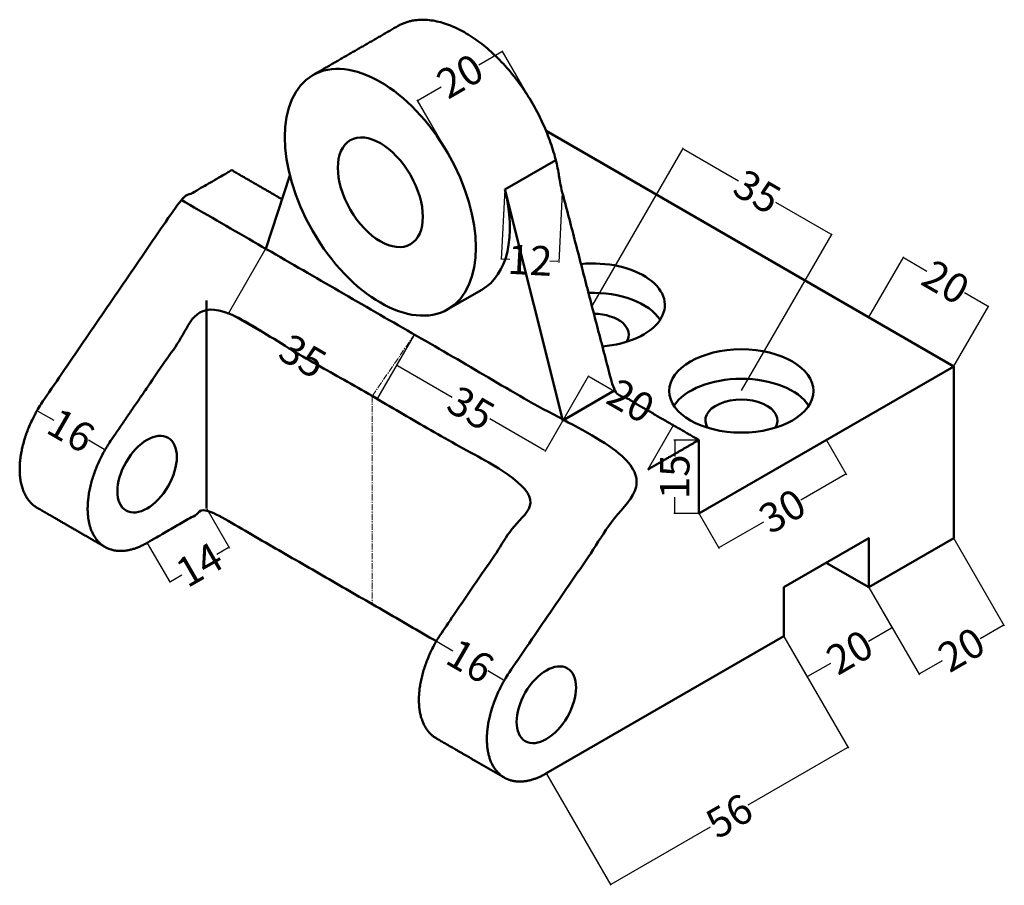
# Model space of a CAD drawing. Units: millimetres. Extents: x 17 to 218, y -59 to 117.
import ezdxf

# ---------------------------------------------------------------- set-up
doc = ezdxf.new("R2010")
doc.units = ezdxf.units.MM
doc.header["$MEASUREMENT"] = 0
doc.linetypes.add('CENTER', pattern=[2, 1.25, -0.25, 0.25, -0.25])
for name, color, linetype, lineweight in [('M-CNTR', 4, 'CENTER', 18), ('M-DIMS', 2, 'Continuous', 25), ('M-OUTL', 7, 'Continuous', 50)]:
    doc.layers.add(name, color=color, linetype=linetype, lineweight=lineweight)
doc.styles.get("Standard").update_dxf_attribs({"font": 'arial.ttf'})
doc.dimstyles.get("Standard").update_dxf_attribs({"dimtxt": 6, "dimasz": 0.18, "dimexe": 0.18, "dimexo": 0.0625, "dimgap": 0.09, "dimtad": 0, "dimtoh": 1, "dimdec": 0, "dimzin": 0, "dimdsep": 46, "dimtxsty": 'Standard', "dimcen": 0.09, "dimadec": 0, "dimazin": 0, "dimtfac": 1, "dimtdec": 0, "dimtofl": 0, "dimtmove": 0, "dimatfit": 3, "dimfxl": 1, "dimtolj": 1, "dimtzin": 0, "dimarcsym": 0})

# ---------------------------------------------------------------- blocks, each defined once
blk = doc.blocks.new('*D1')
at = {"layer": 'Defpoints', "color": 0, "transparency": 16777216}
for p in [(115.95, 82.7), (127.69, 82.09), (126.94, 67.95)]:
    blk.add_point(p, dxfattribs=at)
at = {"layer": 'M-DIMS', "color": 0, "lineweight": -2, "transparency": 16777216}
for p, q in [((115.95, 82.64), (115.2, 68.39)), ((127.68, 82.03), (126.94, 67.77)), ((115.39, 68.56), (117.01, 68.47)), ((126.77, 67.96), (125.14, 68.05))]:
    blk.add_line(p, q, dxfattribs=at)
at = {"layer": 'M-DIMS', "color": 0, "transparency": 16777216}
for points in [[(115.39, 68.59), (115.39, 68.53), (115.21, 68.57)], [(126.77, 67.99), (126.76, 67.93), (126.94, 67.95)]]:
    blk.add_solid(points, dxfattribs=at)
at = {"layer": 'M-DIMS', "color": 0, "transparency": 16777216, "insert": (121.08, 68.26), "char_height": 6, "attachment_point": 5, "rotation": 356.9969}
blk.add_mtext('\\A1;12', dxfattribs=at)
blk = doc.blocks.new('*D2')
at = {"layer": 'Defpoints', "color": 0, "transparency": 16777216}
for p in [(67.19, 70.6), (97.5, 53.1), (89.91, 39.95)]:
    blk.add_point(p, dxfattribs=at)
at = {"layer": 'M-DIMS', "color": 0, "lineweight": -2, "transparency": 16777216}
for p, q in [((67.16, 70.55), (59.51, 57.3)), ((59.76, 57.36), (70.94, 50.91)), ((97.47, 53.05), (89.82, 39.8)), ((89.75, 40.04), (78.57, 46.5))]:
    blk.add_line(p, q, dxfattribs=at)
at = {"layer": 'M-DIMS', "color": 0, "transparency": 16777216}
for points in [[(59.77, 57.39), (59.74, 57.34), (59.6, 57.45)], [(89.77, 40.07), (89.74, 40.02), (89.91, 39.95)]]:
    blk.add_solid(points, dxfattribs=at)
at = {"layer": 'M-DIMS', "color": 0, "transparency": 16777216, "insert": (74.76, 48.7), "char_height": 6, "attachment_point": 5, "rotation": 330}
blk.add_mtext('\\A1;35', dxfattribs=at)
blk = doc.blocks.new('*D3')
at = {"layer": 'Defpoints', "color": 0, "transparency": 16777216}
for p in [(97.5, 53.1), (127.81, 35.6), (124.21, 29.37)]:
    blk.add_point(p, dxfattribs=at)
at = {"layer": 'M-DIMS', "color": 0, "lineweight": -2, "transparency": 16777216}
for p, q in [((97.47, 53.05), (93.81, 46.71)), ((94.06, 46.78), (105.24, 40.32)), ((124.06, 29.46), (112.87, 35.91)), ((127.78, 35.55), (124.12, 29.21))]:
    blk.add_line(p, q, dxfattribs=at)
at = {"layer": 'M-DIMS', "color": 0, "transparency": 16777216}
for points in [[(94.07, 46.8), (94.04, 46.75), (93.9, 46.87)], [(124.07, 29.48), (124.04, 29.43), (124.21, 29.37)]]:
    blk.add_solid(points, dxfattribs=at)
at = {"layer": 'M-DIMS', "color": 0, "transparency": 16777216, "insert": (109.06, 38.12), "char_height": 6, "attachment_point": 5, "rotation": 330}
blk.add_mtext('\\A1;35', dxfattribs=at)
blk = doc.blocks.new('*D4')
at = {"layer": 'Defpoints', "color": 0, "transparency": 16777216}
for p in [(115.47, 110.8), (121.67, 100.06), (104.35, 90.06)]:
    blk.add_point(p, dxfattribs=at)
at = {"layer": 'M-DIMS', "color": 0, "lineweight": -2, "transparency": 16777216}
for p, q in [((115.32, 110.71), (110.65, 108.01)), ((121.64, 100.11), (115.38, 110.95)), ((98.31, 100.89), (102.98, 103.58)), ((104.32, 90.11), (98.06, 100.95))]:
    blk.add_line(p, q, dxfattribs=at)
at = {"layer": 'M-DIMS', "color": 0, "transparency": 16777216}
for points in [[(115.3, 110.73), (115.33, 110.68), (115.47, 110.8)], [(98.29, 100.91), (98.32, 100.86), (98.15, 100.8)]]:
    blk.add_solid(points, dxfattribs=at)
at = {"layer": 'M-DIMS', "color": 0, "transparency": 16777216, "insert": (106.81, 105.8), "char_height": 6, "attachment_point": 5, "rotation": 30}
blk.add_mtext('\\A1;20', dxfattribs=at)
blk = doc.blocks.new('*D5')
at = {"layer": 'Defpoints', "color": 0, "transparency": 16777216}
for p in [(127.81, 35.6), (150.33, 34.6), (145.13, 25.6)]:
    blk.add_point(p, dxfattribs=at)
at = {"layer": 'M-DIMS', "color": 0, "lineweight": -2, "transparency": 16777216}
for p, q in [((127.84, 35.66), (133.11, 44.76)), ((133.17, 44.52), (137.84, 41.82)), ((150.18, 34.69), (145.51, 37.39)), ((145.16, 25.65), (150.42, 34.76))]:
    blk.add_line(p, q, dxfattribs=at)
at = {"layer": 'M-DIMS', "color": 0, "transparency": 16777216}
for points in [[(133.19, 44.54), (133.16, 44.49), (133.02, 44.61)], [(150.19, 34.72), (150.16, 34.67), (150.33, 34.6)]]:
    blk.add_solid(points, dxfattribs=at)
at = {"layer": 'M-DIMS', "color": 0, "transparency": 16777216, "insert": (141.67, 39.6), "char_height": 6, "attachment_point": 5, "rotation": 329.9782}
blk.add_mtext('\\A1;20', dxfattribs=at)
blk = doc.blocks.new('*D6')
at = {"layer": 'Defpoints', "color": 0, "transparency": 16777216}
for p in [(172.85, -8.4), (185.92, -31.05), (124.42, -36.36)]:
    blk.add_point(p, dxfattribs=at)
at = {"layer": 'M-DIMS', "color": 0, "lineweight": -2, "transparency": 16777216}
for p, q in [((172.88, -8.45), (186.01, -31.2)), ((185.77, -31.14), (165.51, -42.83)), ((124.45, -36.41), (137.58, -59.16)), ((137.65, -58.92), (157.91, -47.22))]:
    blk.add_line(p, q, dxfattribs=at)
at = {"layer": 'M-DIMS', "color": 0, "transparency": 16777216}
for points in [[(185.75, -31.11), (185.78, -31.16), (185.92, -31.05)], [(137.64, -58.89), (137.67, -58.94), (137.49, -59.01)]]:
    blk.add_solid(points, dxfattribs=at)
at = {"layer": 'M-DIMS', "color": 0, "transparency": 16777216, "insert": (161.71, -45.03), "char_height": 6, "attachment_point": 5, "rotation": 30.0002}
blk.add_mtext('\\A1;56', dxfattribs=at)
blk = doc.blocks.new('*D7')
at = {"layer": 'Defpoints', "color": 0, "transparency": 16777216}
for p in [(190.17, 1.6), (194.93, -6.65), (172.85, -8.4)]:
    blk.add_point(p, dxfattribs=at)
at = {"layer": 'M-DIMS', "color": 0, "lineweight": -2, "transparency": 16777216}
for p, q in [((190.2, 1.55), (195.02, -6.81)), ((194.78, -6.74), (190.11, -9.44)), ((172.88, -8.45), (177.7, -16.81)), ((177.77, -16.56), (182.44, -13.87))]:
    blk.add_line(p, q, dxfattribs=at)
at = {"layer": 'M-DIMS', "color": 0, "transparency": 16777216}
for points in [[(194.76, -6.72), (194.79, -6.77), (194.93, -6.65)], [(177.76, -16.54), (177.79, -16.59), (177.61, -16.65)]]:
    blk.add_solid(points, dxfattribs=at)
at = {"layer": 'M-DIMS', "color": 0, "transparency": 16777216, "insert": (186.27, -11.65), "char_height": 6, "attachment_point": 5, "rotation": 30}
blk.add_mtext('\\A1;20', dxfattribs=at)
blk = doc.blocks.new('*D8')
at = {"layer": 'Defpoints', "color": 0, "transparency": 16777216}
for p in [(207.49, 11.6), (190.17, 1.6), (217.72, -6.11)]:
    blk.add_point(p, dxfattribs=at)
at = {"layer": 'M-DIMS', "color": 0, "lineweight": -2, "transparency": 16777216}
for p, q in [((207.52, 11.55), (217.81, -6.27)), ((190.2, 1.55), (200.49, -16.27)), ((217.56, -6.2), (212.89, -8.9)), ((200.55, -16.02), (205.22, -13.33))]:
    blk.add_line(p, q, dxfattribs=at)
at = {"layer": 'M-DIMS', "color": 0, "transparency": 16777216}
for points in [[(217.55, -6.18), (217.58, -6.23), (217.72, -6.11)], [(200.54, -16), (200.57, -16.05), (200.4, -16.11)]]:
    blk.add_solid(points, dxfattribs=at)
at = {"layer": 'M-DIMS', "color": 0, "transparency": 16777216, "insert": (209.06, -11.11), "char_height": 6, "attachment_point": 5, "rotation": 30}
blk.add_mtext('\\A1;20', dxfattribs=at)
blk = doc.blocks.new('*D9')
at = {"layer": 'Defpoints', "color": 0, "transparency": 16777216}
for p in [(155.53, 31.6), (150.61, 16.6), (155.53, 16.6)]:
    blk.add_point(p, dxfattribs=at)
at = {"layer": 'M-DIMS', "color": 0, "lineweight": -2, "transparency": 16777216}
for p, q in [((155.46, 31.6), (150.43, 31.6)), ((150.61, 31.42), (150.61, 28.23)), ((150.61, 16.78), (150.61, 19.98)), ((155.46, 16.6), (150.43, 16.6))]:
    blk.add_line(p, q, dxfattribs=at)
at = {"layer": 'M-DIMS', "color": 0, "transparency": 16777216}
for points in [[(150.58, 31.42), (150.64, 31.42), (150.61, 31.6)], [(150.58, 16.78), (150.64, 16.78), (150.61, 16.6)]]:
    blk.add_solid(points, dxfattribs=at)
at = {"layer": 'M-DIMS', "color": 0, "transparency": 16777216, "insert": (150.61, 24.1), "char_height": 6, "attachment_point": 5, "rotation": 90}
blk.add_mtext('\\A1;15', dxfattribs=at)
blk = doc.blocks.new('*D10')
at = {"layer": 'Defpoints', "color": 0, "transparency": 16777216}
for p in [(55.14, 17.64), (43.01, 10.64), (47.6, 2.7)]:
    blk.add_point(p, dxfattribs=at)
at = {"layer": 'M-DIMS', "color": 0, "lineweight": -2, "transparency": 16777216}
for p, q in [((55.17, 17.59), (59.81, 9.54)), ((43.04, 10.59), (47.69, 2.54)), ((59.57, 9.61), (57.21, 8.24)), ((47.76, 2.79), (50.12, 4.15))]:
    blk.add_line(p, q, dxfattribs=at)
at = {"layer": 'M-DIMS', "color": 0, "transparency": 16777216}
for points in [[(59.55, 9.63), (59.58, 9.58), (59.72, 9.7)], [(47.74, 2.81), (47.77, 2.76), (47.6, 2.7)]]:
    blk.add_solid(points, dxfattribs=at)
at = {"layer": 'M-DIMS', "color": 0, "transparency": 16777216, "insert": (53.66, 6.2), "char_height": 6, "attachment_point": 5, "rotation": 30}
blk.add_mtext('\\A1;14', dxfattribs=at)
blk = doc.blocks.new('*D11')
at = {"layer": 'Defpoints', "color": 0, "transparency": 16777216}
for p in [(101.99, -9.41), (115.84, -17.41), (115.84, -17.41)]:
    blk.add_point(p, dxfattribs=at)
at = {"layer": 'M-DIMS', "color": 0, "lineweight": -2, "transparency": 16777216}
for p, q in [((102.02, -9.35), (102.08, -9.25)), ((102.14, -9.5), (105.36, -11.36)), ((115.69, -17.32), (112.47, -15.46)), ((115.88, -17.35), (115.93, -17.25))]:
    blk.add_line(p, q, dxfattribs=at)
at = {"layer": 'M-DIMS', "color": 0, "transparency": 16777216}
for points in [[(102.16, -9.47), (102.13, -9.52), (101.99, -9.41)], [(115.7, -17.29), (115.67, -17.34), (115.84, -17.41)]]:
    blk.add_solid(points, dxfattribs=at)
at = {"layer": 'M-DIMS', "color": 0, "transparency": 16777216, "insert": (108.92, -13.41), "char_height": 6, "attachment_point": 5, "rotation": 330}
blk.add_mtext('\\A1;16', dxfattribs=at)
blk = doc.blocks.new('*D12')
at = {"layer": 'Defpoints', "color": 0, "transparency": 16777216}
for p in [(20.58, 37.59), (34.44, 29.59), (34.44, 29.59)]:
    blk.add_point(p, dxfattribs=at)
at = {"layer": 'M-DIMS', "color": 0, "lineweight": -2, "transparency": 16777216}
for p, q in [((20.61, 37.65), (20.67, 37.75)), ((20.74, 37.5), (23.96, 35.64)), ((34.28, 29.68), (31.06, 31.54)), ((34.47, 29.65), (34.53, 29.75))]:
    blk.add_line(p, q, dxfattribs=at)
at = {"layer": 'M-DIMS', "color": 0, "transparency": 16777216}
for points in [[(20.75, 37.53), (20.72, 37.48), (20.58, 37.59)], [(34.3, 29.71), (34.27, 29.66), (34.44, 29.59)]]:
    blk.add_solid(points, dxfattribs=at)
at = {"layer": 'M-DIMS', "color": 0, "transparency": 16777216, "insert": (27.51, 33.59), "char_height": 6, "attachment_point": 5, "rotation": 330}
blk.add_mtext('\\A1;16', dxfattribs=at)
blk = doc.blocks.new('*D13')
at = {"layer": 'Defpoints', "color": 0, "transparency": 16777216}
for p in [(182.59, 73.48), (133.88, 59.1), (164.19, 41.6)]:
    blk.add_point(p, dxfattribs=at)
at = {"layer": 'M-DIMS', "color": 0, "lineweight": -2, "transparency": 16777216}
for p, q in [((133.91, 59.16), (152.37, 91.14)), ((152.44, 90.89), (163.62, 84.43)), ((182.43, 73.57), (171.25, 80.03)), ((164.22, 41.66), (182.68, 73.64))]:
    blk.add_line(p, q, dxfattribs=at)
at = {"layer": 'M-DIMS', "color": 0, "transparency": 16777216}
for points in [[(152.45, 90.92), (152.42, 90.86), (152.28, 90.98)], [(182.45, 73.6), (182.42, 73.54), (182.59, 73.48)]]:
    blk.add_solid(points, dxfattribs=at)
at = {"layer": 'M-DIMS', "color": 0, "transparency": 16777216, "insert": (167.43, 82.23), "char_height": 6, "attachment_point": 5, "rotation": 330}
blk.add_mtext('\\A1;35', dxfattribs=at)
blk = doc.blocks.new('*D14')
at = {"layer": 'Defpoints', "color": 0, "transparency": 16777216}
for p in [(181.51, 31.6), (185.53, 24.64), (155.53, 16.6)]:
    blk.add_point(p, dxfattribs=at)
at = {"layer": 'M-DIMS', "color": 0, "lineweight": -2, "transparency": 16777216}
for p, q in [((181.54, 31.55), (185.62, 24.48)), ((185.37, 24.55), (176.33, 19.32)), ((155.56, 16.55), (159.64, 9.48)), ((159.7, 9.73), (168.75, 14.95))]:
    blk.add_line(p, q, dxfattribs=at)
at = {"layer": 'M-DIMS', "color": 0, "transparency": 16777216}
for points in [[(185.36, 24.57), (185.39, 24.52), (185.53, 24.64)], [(159.69, 9.75), (159.72, 9.7), (159.55, 9.64)]]:
    blk.add_solid(points, dxfattribs=at)
at = {"layer": 'M-DIMS', "color": 0, "transparency": 16777216, "insert": (172.54, 17.14), "char_height": 6, "attachment_point": 5, "rotation": 30}
blk.add_mtext('\\A1;30', dxfattribs=at)
blk = doc.blocks.new('*D15')
at = {"layer": 'Defpoints', "color": 0, "transparency": 16777216}
for p in [(197.21, 68.8), (190.17, 56.6), (207.49, 46.6)]:
    blk.add_point(p, dxfattribs=at)
at = {"layer": 'M-DIMS', "color": 0, "lineweight": -2, "transparency": 16777216}
for p, q in [((190.2, 56.66), (197.3, 68.96)), ((197.37, 68.71), (202.03, 66.01)), ((214.37, 58.89), (209.7, 61.59)), ((207.52, 46.66), (214.62, 58.96))]:
    blk.add_line(p, q, dxfattribs=at)
at = {"layer": 'M-DIMS', "color": 0, "transparency": 16777216}
for points in [[(197.38, 68.74), (197.35, 68.68), (197.21, 68.8)], [(214.39, 58.92), (214.36, 58.86), (214.53, 58.8)]]:
    blk.add_solid(points, dxfattribs=at)
at = {"layer": 'M-DIMS', "color": 0, "transparency": 16777216, "insert": (205.87, 63.8), "char_height": 6, "attachment_point": 5, "rotation": 330}
blk.add_mtext('\\A1;20', dxfattribs=at)

msp = doc.modelspace()

# ---------------------------------------------------------------- linework, layer by layer
at = {"layer": 'M-CNTR'}
msp.add_lwpolyline([(97.57, 53.2), (88.91, 40.53), (88.91, -1.86)], dxfattribs=at)
at = {"layer": 'M-OUTL'}
for p, q in [((115.96, 82.67), (126.35, 88.67)), ((67.19, 70.6), (72.13, 85.49)), ((127.81, 35.6), (115.95, 82.7)), ((76.1, 75.4), (76.1, 75.4)), ((104.35, 58.24), (111.28, 62.24)), ((55.14, 60.03), (55.14, 17.64)), ((138.21, 41.6), (127.81, 35.6)), ((136.54, -29.36), (136.54, -29.36))]:
    msp.add_line(p, q, dxfattribs=at)
for points in [[(155.53, 31.6), (155.53, 16.6), (207.49, 46.6), (124.38, 94.59)], [(190.17, 1.6), (207.49, 11.6), (207.49, 46.6)], [(124.35, -36.4), (172.85, -8.4), (172.85, 1.6), (190.17, 11.6), (190.17, 1.6), (181.51, 6.6)]]:
    msp.add_lwpolyline(points, dxfattribs=at)
for centre, major_axis in [((90.57, 82.1), (13.78, -23.86)), ((90.57, 82.1), (6.12, -10.61)), ((164.19, 41.6), (-14.7, 0)), ((43.01, 24.64), (-4.29, -7.42)), ((124.42, -22.36), (-4.29, -7.42))]:
    msp.add_ellipse(centre, major_axis=major_axis, ratio=0.57735, dxfattribs=at)
for centre, major_axis, start_param, end_param in [((97.5, 86.1), (13.78, -23.86), 6.283185, 7.396657), ((133.88, 59.1), (-14.7, 0), 1.705098, 4.875904), ((133.88, 53.1), (-14.7, 0), 3.50296, 4.770875), ((133.88, 53.1), (-7.35, 0), 2.780226, 4.679703), ((164.19, 35.6), (-14.7, 0), 3.50296, 5.921818), ((29.16, 32.64), (-8.57, -14.85), 2.356194, 2.364148), ((164.19, 35.6), (-7.35, 0), 2.780226, 6.644552), ((110.56, -14.36), (-8.57, -14.85), 2.356194, 2.364148)]:
    msp.add_ellipse(centre, major_axis=major_axis, ratio=0.57735, start_param=start_param, end_param=end_param, dxfattribs=at)
for points, weights, knots in [([(145.13, 25.6), (150.33, 28.6), (155.53, 31.6), (146.87, 36.6), (138.21, 41.6), (132.71, 62.76), (127.21, 83.92), (125.61, 98.7), (114.15, 109.81), (102.68, 120.91), (94.12, 115.97), (85.46, 110.97), (76.8, 105.97)], [1, 1, 1, 1, 1, 1, 1, 0.849390997232, 1, 0.849390997232, 1, 1, 1], [0, 0, 0, 1, 1, 2, 2, 3, 3, 4.111932, 4.111932, 5.223864, 5.223864, 6.223864, 6.223864, 6.223864]), ([(70.53, 80.67), (65.4, 83.64), (60.26, 86.6), (55.07, 83.6), (49.87, 80.6), (35.82, 60.05), (21.77, 39.49), (17.42, 33.11), (17.06, 26.57), (16.7, 20.04), (20.58, 17.79), (27.51, 13.79), (34.44, 9.79)], [1, 1, 1, 1, 1, 1, 1, 0.910861092427, 1, 0.910861092427, 1, 1, 1], [0, 0, 0, 1, 1, 2, 2, 3, 3, 3.850861, 3.850861, 4.701723, 4.701723, 5.701723, 5.701723, 5.701723]), ([(49.87, 80.6), (97.5, 53.1), (145.13, 25.6), (131.09, 5.05), (117.04, -15.51), (110.14, -25.6), (112.94, -33.49), (115.73, -41.37), (124.42, -36.36)], [1, 1, 1, 1, 1, 0.812842828072, 1, 0.812842828072, 1], [0, 0, 0, 1, 1, 2, 2, 3.24356, 3.24356, 4.487121, 4.487121, 4.487121]), ([(115.84, -37.21), (108.92, -33.21), (101.99, -29.21), (98.1, -26.96), (98.46, -20.43), (98.82, -13.89), (103.18, -7.51), (112.93, 6.76), (122.69, 21.03), (88.91, 40.53), (55.14, 60.03), (45.38, 45.76), (35.63, 31.49), (28.74, 21.4), (31.53, 13.51), (34.32, 5.63), (43.01, 10.64), (49.07, 14.14), (55.14, 17.64), (78.56, 4.12), (101.99, -9.41)], [1, 1, 1, 0.910861092427, 1, 0.910861092427, 1, 1, 1, 1, 1, 1, 1, 0.812842828072, 1, 0.812842828072, 1, 1, 1, 1, 1], [0, 0, 0, 1, 1, 1.850861, 1.850861, 2.701723, 2.701723, 3.701723, 3.701723, 4.701723, 4.701723, 5.701723, 5.701723, 6.945283, 6.945283, 8.188843, 8.188843, 9.188843, 9.188843, 10.188843, 10.188843, 10.188843])]:
    msp.add_rational_spline(points, weights, degree=2, knots=knots, dxfattribs=at)

# ---------------------------------------------------------------- dimensions: what is measured, and where the dimension line sits
at = {"layer": 'M-DIMS'}
for p1, p2, distance, picture, middle in [((104.35, 90.06), (121.67, 100.06), 12.4, '*D4', (106.81, 105.8)), ((133.88, 59.1), (164.19, 41.6), 36.81, '*D13', (167.43, 82.23)), ((115.95, 82.7), (127.69, 82.09), -14.15, '*D1', (121.08, 68.26)), ((67.19, 70.6), (97.5, 53.1), -15.18, '*D2', (74.76, 48.7)), ((207.49, 46.6), (190.17, 56.6), -14.08, '*D15', (205.87, 63.8)), ((97.5, 53.1), (127.81, 35.6), -7.2, '*D3', (109.06, 38.12)), ((127.81, 35.6), (145.13, 25.6), 10.4, '*D5', (141.67, 39.6)), ((20.58, 37.59), (34.44, 29.59), 0, '*D12', (27.51, 33.59)), ((155.53, 31.6), (155.53, 16.6), -4.91, '*D9', (150.61, 24.1)), ((155.53, 16.6), (181.51, 31.6), -8.04, '*D14', (172.54, 17.14)), ((55.14, 17.64), (43.01, 10.64), 9.18, '*D10', (53.66, 6.2)), ((190.17, 1.6), (207.49, 11.6), -20.46, '*D8', (209.06, -11.11)), ((172.85, -8.4), (190.17, 1.6), -9.54, '*D7', (186.27, -11.65)), ((101.99, -9.41), (115.84, -17.41), 0, '*D11', (108.92, -13.41)), ((124.42, -36.36), (172.85, -8.4), -26.15, '*D6', (161.71, -45.03))]:
    dim = msp.add_aligned_dim(p1=p1, p2=p2, distance=distance, dimstyle='Standard', override={"dimclrd": 0, "dimclre": 0, "dimclrt": 0}, dxfattribs=at)
    dim.commit()
    dim.dimension.update_dxf_attribs({"geometry": picture, "text_midpoint": middle})

doc.saveas('drawing.dxf')
